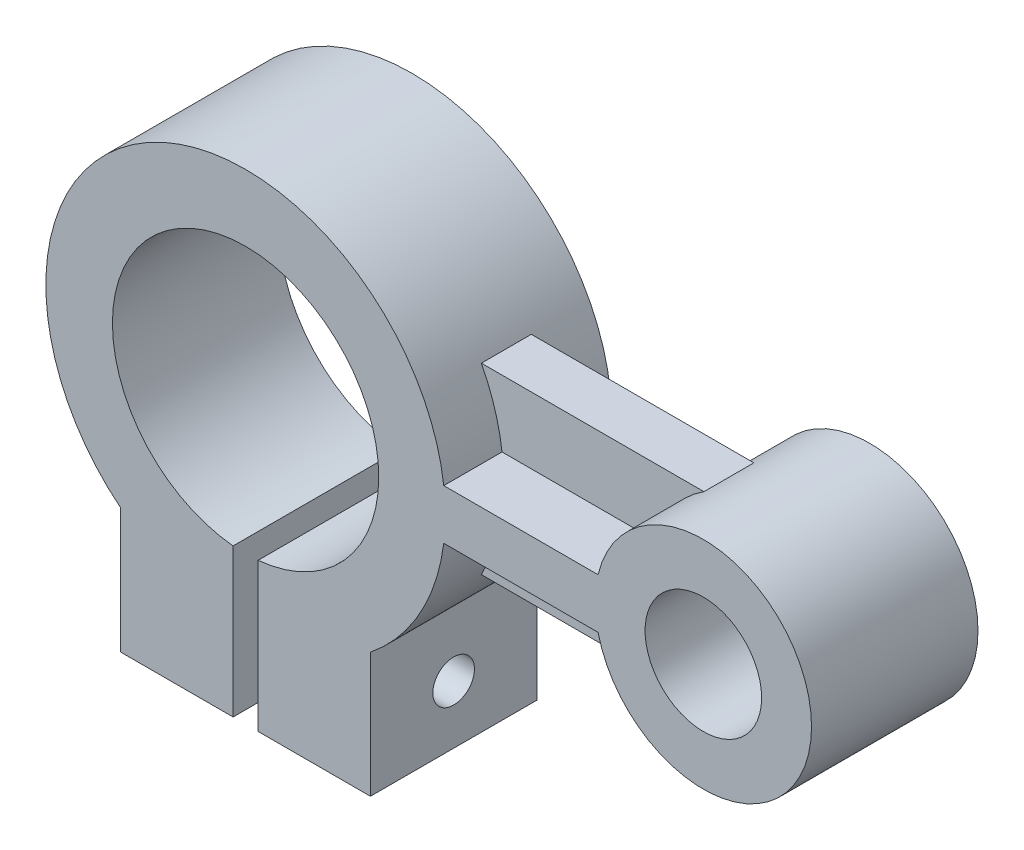
ISO-10303-21;
HEADER;
FILE_DESCRIPTION(('STEP AP214'),'2;1');
FILE_NAME('part.step','',(''),(''),'','','');
FILE_SCHEMA(('AUTOMOTIVE_DESIGN { 1 0 10303 214 1 1 1 1 }'));
ENDSEC;
DATA;
#1=APPLICATION_CONTEXT('core data for automotive mechanical design processes');
#2=APPLICATION_PROTOCOL_DEFINITION('international standard','automotive_design',2000,#1);
#3=PRODUCT_CONTEXT('',#1,'mechanical');
#4=PRODUCT('Part','Part','',(#3));
#5=PRODUCT_RELATED_PRODUCT_CATEGORY('part','',(#4));
#6=PRODUCT_DEFINITION_FORMATION('','',#4);
#7=PRODUCT_DEFINITION_CONTEXT('part definition',#1,'design');
#8=PRODUCT_DEFINITION('design','',#6,#7);
#9=PRODUCT_DEFINITION_SHAPE('','',#8);
#10=(LENGTH_UNIT() NAMED_UNIT(*) SI_UNIT(.MILLI.,.METRE.));
#11=(NAMED_UNIT(*) PLANE_ANGLE_UNIT() SI_UNIT($,.RADIAN.));
#12=(NAMED_UNIT(*) SI_UNIT($,.STERADIAN.) SOLID_ANGLE_UNIT());
#13=UNCERTAINTY_MEASURE_WITH_UNIT(LENGTH_MEASURE(1.E-05),#10,'distance_accuracy_value','');
#14=(GEOMETRIC_REPRESENTATION_CONTEXT(3) GLOBAL_UNCERTAINTY_ASSIGNED_CONTEXT((#13)) GLOBAL_UNIT_ASSIGNED_CONTEXT((#10,
#11,#12)) REPRESENTATION_CONTEXT('',''));
#15=CARTESIAN_POINT('',(0.,0.,0.));
#16=DIRECTION('',(0.,0.,1.));
#17=DIRECTION('',(1.,0.,0.));
#18=AXIS2_PLACEMENT_3D('',#15,#16,#17);
#19=CARTESIAN_POINT('',(110.,0.,0.));
#20=DIRECTION('',(0.,0.,1.));
#21=DIRECTION('',(1.,0.,0.));
#22=AXIS2_PLACEMENT_3D('',#19,#20,#21);
#23=CYLINDRICAL_SURFACE('',#22,26.);
#24=DIRECTION('',(0.,0.,1.));
#25=VECTOR('',#24,1.);
#26=CARTESIAN_POINT('',(96.143593539449,-22.,0.));
#27=LINE('',#26,#25);
#28=CARTESIAN_POINT('',(96.143593539449,-22.,26.));
#29=VERTEX_POINT('',#28);
#30=CARTESIAN_POINT('',(96.143593539449,-22.,14.));
#31=VERTEX_POINT('',#30);
#32=EDGE_CURVE('E345',#29,#31,#27,.F.);
#33=ORIENTED_EDGE('',*,*,#32,.T.);
#34=CARTESIAN_POINT('',(110.,0.,14.));
#35=DIRECTION('',(0.,0.,1.));
#36=DIRECTION('',(1.,0.,0.));
#37=AXIS2_PLACEMENT_3D('',#34,#35,#36);
#38=CIRCLE('',#37,26.);
#39=CARTESIAN_POINT('',(84.701778718653,-6.,14.));
#40=VERTEX_POINT('',#39);
#41=EDGE_CURVE('E349',#31,#40,#38,.F.);
#42=ORIENTED_EDGE('',*,*,#41,.T.);
#43=DIRECTION('',(0.,0.,1.));
#44=VECTOR('',#43,1.);
#45=CARTESIAN_POINT('',(84.701778718653,-6.,0.));
#46=LINE('',#45,#44);
#47=CARTESIAN_POINT('',(84.701778718653,-6.,0.));
#48=VERTEX_POINT('',#47);
#49=EDGE_CURVE('E214',#48,#40,#46,.T.);
#50=ORIENTED_EDGE('',*,*,#49,.F.);
#51=CARTESIAN_POINT('',(110.,0.,0.));
#52=DIRECTION('',(0.,0.,1.));
#53=DIRECTION('',(1.,0.,0.));
#54=AXIS2_PLACEMENT_3D('',#51,#52,#53);
#55=CIRCLE('',#54,26.);
#56=CARTESIAN_POINT('',(84.701778718653,6.,0.));
#57=VERTEX_POINT('',#56);
#58=EDGE_CURVE('E309',#48,#57,#55,.T.);
#59=ORIENTED_EDGE('',*,*,#58,.T.);
#60=DIRECTION('',(0.,0.,1.));
#61=VECTOR('',#60,1.);
#62=CARTESIAN_POINT('',(84.701778718653,6.,0.));
#63=LINE('',#62,#61);
#64=CARTESIAN_POINT('',(84.701778718653,6.,14.));
#65=VERTEX_POINT('',#64);
#66=EDGE_CURVE('E217',#57,#65,#63,.T.);
#67=ORIENTED_EDGE('',*,*,#66,.T.);
#68=CARTESIAN_POINT('',(110.,0.,14.));
#69=DIRECTION('',(0.,0.,1.));
#70=DIRECTION('',(1.,0.,0.));
#71=AXIS2_PLACEMENT_3D('',#68,#69,#70);
#72=CIRCLE('',#71,26.);
#73=CARTESIAN_POINT('',(96.143593539449,22.,14.));
#74=VERTEX_POINT('',#73);
#75=EDGE_CURVE('E286',#65,#74,#72,.F.);
#76=ORIENTED_EDGE('',*,*,#75,.T.);
#77=DIRECTION('',(0.,0.,1.));
#78=VECTOR('',#77,1.);
#79=CARTESIAN_POINT('',(96.143593539449,22.,0.));
#80=LINE('',#79,#78);
#81=CARTESIAN_POINT('',(96.143593539449,22.,26.));
#82=VERTEX_POINT('',#81);
#83=EDGE_CURVE('E278',#74,#82,#80,.T.);
#84=ORIENTED_EDGE('',*,*,#83,.T.);
#85=CARTESIAN_POINT('',(110.,0.,26.));
#86=DIRECTION('',(0.,0.,-1.));
#87=DIRECTION('',(-1.,0.,0.));
#88=AXIS2_PLACEMENT_3D('',#85,#86,#87);
#89=CIRCLE('',#88,26.);
#90=CARTESIAN_POINT('',(84.701778718653,6.,26.));
#91=VERTEX_POINT('',#90);
#92=EDGE_CURVE('E188',#82,#91,#89,.F.);
#93=ORIENTED_EDGE('',*,*,#92,.T.);
#94=CARTESIAN_POINT('',(84.701778718653,6.,40.));
#95=VERTEX_POINT('',#94);
#96=EDGE_CURVE('E216',#91,#95,#63,.T.);
#97=ORIENTED_EDGE('',*,*,#96,.T.);
#98=CARTESIAN_POINT('',(110.,0.,40.));
#99=DIRECTION('',(0.,0.,1.));
#100=DIRECTION('',(1.,0.,0.));
#101=AXIS2_PLACEMENT_3D('',#98,#99,#100);
#102=CIRCLE('',#101,26.);
#103=CARTESIAN_POINT('',(84.701778718653,-6.,40.));
#104=VERTEX_POINT('',#103);
#105=EDGE_CURVE('E321',#104,#95,#102,.T.);
#106=ORIENTED_EDGE('',*,*,#105,.F.);
#107=CARTESIAN_POINT('',(84.701778718653,-6.,26.));
#108=VERTEX_POINT('',#107);
#109=EDGE_CURVE('E206',#108,#104,#46,.T.);
#110=ORIENTED_EDGE('',*,*,#109,.F.);
#111=CARTESIAN_POINT('',(110.,0.,26.));
#112=DIRECTION('',(0.,0.,-1.));
#113=DIRECTION('',(-1.,0.,0.));
#114=AXIS2_PLACEMENT_3D('',#111,#112,#113);
#115=CIRCLE('',#114,26.);
#116=EDGE_CURVE('E64',#108,#29,#115,.F.);
#117=ORIENTED_EDGE('',*,*,#116,.T.);
#118=EDGE_LOOP('',(#33,#42,#50,#59,#67,#76,#84,#93,#97,#106,#110,#117));
#119=FACE_BOUND('',#118,.T.);
#120=ADVANCED_FACE('F50',(#119),#23,.T.);
#121=CARTESIAN_POINT('',(0.,0.,40.));
#122=DIRECTION('',(0.,0.,-1.));
#123=DIRECTION('',(-1.,0.,0.));
#124=AXIS2_PLACEMENT_3D('',#121,#122,#123);
#125=CYLINDRICAL_SURFACE('',#124,48.);
#126=CARTESIAN_POINT('',(0.,0.,14.));
#127=DIRECTION('',(0.,0.,1.));
#128=DIRECTION('',(1.,0.,0.));
#129=AXIS2_PLACEMENT_3D('',#126,#127,#128);
#130=CIRCLE('',#129,48.);
#131=CARTESIAN_POINT('',(42.6614580154031,-22.,14.));
#132=VERTEX_POINT('',#131);
#133=CARTESIAN_POINT('',(47.6235235991626,-6.,14.));
#134=VERTEX_POINT('',#133);
#135=EDGE_CURVE('E297',#132,#134,#130,.T.);
#136=ORIENTED_EDGE('',*,*,#135,.F.);
#137=DIRECTION('',(0.,0.,-1.));
#138=VECTOR('',#137,1.);
#139=CARTESIAN_POINT('',(42.6614580154031,-22.,40.));
#140=LINE('',#139,#138);
#141=CARTESIAN_POINT('',(42.6614580154031,-22.,26.));
#142=VERTEX_POINT('',#141);
#143=EDGE_CURVE('E11',#142,#132,#140,.T.);
#144=ORIENTED_EDGE('',*,*,#143,.F.);
#145=CARTESIAN_POINT('',(0.,0.,26.));
#146=DIRECTION('',(0.,0.,-1.));
#147=DIRECTION('',(-1.,0.,0.));
#148=AXIS2_PLACEMENT_3D('',#145,#146,#147);
#149=CIRCLE('',#148,48.);
#150=CARTESIAN_POINT('',(47.6235235991626,-6.,26.));
#151=VERTEX_POINT('',#150);
#152=EDGE_CURVE('E184',#151,#142,#149,.T.);
#153=ORIENTED_EDGE('',*,*,#152,.F.);
#154=DIRECTION('',(0.,0.,1.));
#155=VECTOR('',#154,1.);
#156=CARTESIAN_POINT('',(47.6235235991626,-6.00000000000002,0.));
#157=LINE('',#156,#155);
#158=CARTESIAN_POINT('',(47.6235235991626,-6.00000000000001,40.));
#159=VERTEX_POINT('',#158);
#160=EDGE_CURVE('E197',#151,#159,#157,.T.);
#161=ORIENTED_EDGE('',*,*,#160,.T.);
#162=CARTESIAN_POINT('',(0.,0.,40.));
#163=DIRECTION('',(0.,0.,1.));
#164=DIRECTION('',(1.,0.,0.));
#165=AXIS2_PLACEMENT_3D('',#162,#163,#164);
#166=CIRCLE('',#165,48.);
#167=CARTESIAN_POINT('',(30.,-37.4699879903904,40.));
#168=VERTEX_POINT('',#167);
#169=EDGE_CURVE('E279',#168,#159,#166,.T.);
#170=ORIENTED_EDGE('',*,*,#169,.F.);
#171=DIRECTION('',(0.,0.,1.));
#172=VECTOR('',#171,1.);
#173=CARTESIAN_POINT('',(30.,-37.4699879903904,0.));
#174=LINE('',#173,#172);
#175=CARTESIAN_POINT('',(30.,-37.4699879903904,0.));
#176=VERTEX_POINT('',#175);
#177=EDGE_CURVE('E267',#176,#168,#174,.T.);
#178=ORIENTED_EDGE('',*,*,#177,.F.);
#179=CARTESIAN_POINT('',(0.,0.,0.));
#180=DIRECTION('',(0.,0.,1.));
#181=DIRECTION('',(1.,0.,0.));
#182=AXIS2_PLACEMENT_3D('',#179,#180,#181);
#183=CIRCLE('',#182,48.);
#184=CARTESIAN_POINT('',(47.6235235991626,-6.00000000000001,0.));
#185=VERTEX_POINT('',#184);
#186=EDGE_CURVE('E284',#176,#185,#183,.T.);
#187=ORIENTED_EDGE('',*,*,#186,.T.);
#188=EDGE_CURVE('E203',#185,#134,#157,.T.);
#189=ORIENTED_EDGE('',*,*,#188,.T.);
#190=EDGE_LOOP('',(#136,#144,#153,#161,#170,#178,#187,#189));
#191=FACE_BOUND('',#190,.T.);
#192=ADVANCED_FACE('F193',(#191),#125,.T.);
#193=CARTESIAN_POINT('',(47.6235235991626,-6.,0.));
#194=DIRECTION('',(0.,-1.,0.));
#195=DIRECTION('',(1.,0.,0.));
#196=AXIS2_PLACEMENT_3D('',#193,#194,#195);
#197=PLANE('',#196);
#198=ORIENTED_EDGE('',*,*,#49,.T.);
#199=DIRECTION('',(-1.,0.,0.));
#200=VECTOR('',#199,1.);
#201=CARTESIAN_POINT('',(47.6235235991626,-6.,14.));
#202=LINE('',#201,#200);
#203=EDGE_CURVE('E57',#40,#134,#202,.T.);
#204=ORIENTED_EDGE('',*,*,#203,.T.);
#205=ORIENTED_EDGE('',*,*,#188,.F.);
#206=DIRECTION('',(1.,0.,0.));
#207=VECTOR('',#206,1.);
#208=CARTESIAN_POINT('',(47.6235235991626,-6.,0.));
#209=LINE('',#208,#207);
#210=EDGE_CURVE('E310',#185,#48,#209,.T.);
#211=ORIENTED_EDGE('',*,*,#210,.T.);
#212=EDGE_LOOP('',(#198,#204,#205,#211));
#213=FACE_BOUND('',#212,.T.);
#214=ADVANCED_FACE('F294',(#213),#197,.T.);
#215=ORIENTED_EDGE('',*,*,#160,.F.);
#216=DIRECTION('',(1.,0.,0.));
#217=VECTOR('',#216,1.);
#218=CARTESIAN_POINT('',(47.6235235991626,-6.,26.));
#219=LINE('',#218,#217);
#220=EDGE_CURVE('E185',#151,#108,#219,.T.);
#221=ORIENTED_EDGE('',*,*,#220,.T.);
#222=ORIENTED_EDGE('',*,*,#109,.T.);
#223=DIRECTION('',(1.,0.,0.));
#224=VECTOR('',#223,1.);
#225=CARTESIAN_POINT('',(47.6235235991626,-6.,40.));
#226=LINE('',#225,#224);
#227=EDGE_CURVE('E204',#159,#104,#226,.T.);
#228=ORIENTED_EDGE('',*,*,#227,.F.);
#229=EDGE_LOOP('',(#215,#221,#222,#228));
#230=FACE_BOUND('',#229,.T.);
#231=ADVANCED_FACE('F201',(#230),#197,.T.);
#232=CARTESIAN_POINT('',(0.,0.,26.));
#233=DIRECTION('',(0.,0.,-1.));
#234=DIRECTION('',(-1.,0.,0.));
#235=AXIS2_PLACEMENT_3D('',#232,#233,#234);
#236=CIRCLE('',#235,48.);
#237=CARTESIAN_POINT('',(42.6614580154031,22.,26.));
#238=VERTEX_POINT('',#237);
#239=CARTESIAN_POINT('',(47.6235235991626,6.,26.));
#240=VERTEX_POINT('',#239);
#241=EDGE_CURVE('E326',#238,#240,#236,.T.);
#242=ORIENTED_EDGE('',*,*,#241,.F.);
#243=DIRECTION('',(0.,0.,-1.));
#244=VECTOR('',#243,1.);
#245=CARTESIAN_POINT('',(42.6614580154031,22.,40.));
#246=LINE('',#245,#244);
#247=CARTESIAN_POINT('',(42.6614580154031,22.,14.));
#248=VERTEX_POINT('',#247);
#249=EDGE_CURVE('E335',#248,#238,#246,.F.);
#250=ORIENTED_EDGE('',*,*,#249,.F.);
#251=CARTESIAN_POINT('',(0.,0.,14.));
#252=DIRECTION('',(0.,0.,1.));
#253=DIRECTION('',(1.,0.,0.));
#254=AXIS2_PLACEMENT_3D('',#251,#252,#253);
#255=CIRCLE('',#254,48.);
#256=CARTESIAN_POINT('',(47.6235235991626,6.,14.));
#257=VERTEX_POINT('',#256);
#258=EDGE_CURVE('E331',#257,#248,#255,.T.);
#259=ORIENTED_EDGE('',*,*,#258,.F.);
#260=DIRECTION('',(0.,0.,1.));
#261=VECTOR('',#260,1.);
#262=CARTESIAN_POINT('',(47.6235235991626,6.,0.));
#263=LINE('',#262,#261);
#264=CARTESIAN_POINT('',(47.6235235991626,6.,0.));
#265=VERTEX_POINT('',#264);
#266=EDGE_CURVE('E205',#265,#257,#263,.T.);
#267=ORIENTED_EDGE('',*,*,#266,.F.);
#268=CARTESIAN_POINT('',(-30.,-37.4699879903904,0.));
#269=VERTEX_POINT('',#268);
#270=EDGE_CURVE('E270',#265,#269,#183,.T.);
#271=ORIENTED_EDGE('',*,*,#270,.T.);
#272=DIRECTION('',(0.,0.,1.));
#273=VECTOR('',#272,1.);
#274=CARTESIAN_POINT('',(-30.,-37.4699879903904,0.));
#275=LINE('',#274,#273);
#276=CARTESIAN_POINT('',(-30.,-37.4699879903904,40.));
#277=VERTEX_POINT('',#276);
#278=EDGE_CURVE('E259',#269,#277,#275,.T.);
#279=ORIENTED_EDGE('',*,*,#278,.T.);
#280=CARTESIAN_POINT('',(47.6235235991626,6.,40.));
#281=VERTEX_POINT('',#280);
#282=EDGE_CURVE('E282',#281,#277,#166,.T.);
#283=ORIENTED_EDGE('',*,*,#282,.F.);
#284=EDGE_CURVE('E208',#240,#281,#263,.T.);
#285=ORIENTED_EDGE('',*,*,#284,.F.);
#286=EDGE_LOOP('',(#242,#250,#259,#267,#271,#279,#283,#285));
#287=FACE_BOUND('',#286,.T.);
#288=ADVANCED_FACE('F47',(#287),#125,.T.);
#289=CARTESIAN_POINT('',(47.6235235991626,6.,0.));
#290=DIRECTION('',(0.,1.,0.));
#291=DIRECTION('',(-1.,0.,0.));
#292=AXIS2_PLACEMENT_3D('',#289,#290,#291);
#293=PLANE('',#292);
#294=ORIENTED_EDGE('',*,*,#96,.F.);
#295=DIRECTION('',(1.,0.,0.));
#296=VECTOR('',#295,1.);
#297=CARTESIAN_POINT('',(110.350889359326,6.,26.));
#298=LINE('',#297,#296);
#299=EDGE_CURVE('E338',#240,#91,#298,.T.);
#300=ORIENTED_EDGE('',*,*,#299,.F.);
#301=ORIENTED_EDGE('',*,*,#284,.T.);
#302=DIRECTION('',(-1.,0.,0.));
#303=VECTOR('',#302,1.);
#304=CARTESIAN_POINT('',(47.6235235991626,6.,40.));
#305=LINE('',#304,#303);
#306=EDGE_CURVE('E320',#95,#281,#305,.T.);
#307=ORIENTED_EDGE('',*,*,#306,.F.);
#308=EDGE_LOOP('',(#294,#300,#301,#307));
#309=FACE_BOUND('',#308,.T.);
#310=ADVANCED_FACE('F405',(#309),#293,.T.);
#311=ORIENTED_EDGE('',*,*,#266,.T.);
#312=DIRECTION('',(-1.,0.,0.));
#313=VECTOR('',#312,1.);
#314=CARTESIAN_POINT('',(39.2683528470453,6.,14.));
#315=LINE('',#314,#313);
#316=EDGE_CURVE('E336',#65,#257,#315,.T.);
#317=ORIENTED_EDGE('',*,*,#316,.F.);
#318=ORIENTED_EDGE('',*,*,#66,.F.);
#319=DIRECTION('',(-1.,0.,0.));
#320=VECTOR('',#319,1.);
#321=CARTESIAN_POINT('',(47.6235235991626,6.,0.));
#322=LINE('',#321,#320);
#323=EDGE_CURVE('E311',#57,#265,#322,.T.);
#324=ORIENTED_EDGE('',*,*,#323,.T.);
#325=EDGE_LOOP('',(#311,#317,#318,#324));
#326=FACE_BOUND('',#325,.T.);
#327=ADVANCED_FACE('F403',(#326),#293,.T.);
#328=CARTESIAN_POINT('',(-30.,-67.4699879903904,0.));
#329=DIRECTION('',(0.,-1.,0.));
#330=DIRECTION('',(0.,0.,-1.));
#331=AXIS2_PLACEMENT_3D('',#328,#329,#330);
#332=PLANE('',#331);
#333=DIRECTION('',(0.,0.,1.));
#334=VECTOR('',#333,1.);
#335=CARTESIAN_POINT('',(3.00000000000001,-67.4699879903904,0.));
#336=LINE('',#335,#334);
#337=CARTESIAN_POINT('',(3.00000000000001,-67.4699879903904,0.));
#338=VERTEX_POINT('',#337);
#339=CARTESIAN_POINT('',(3.00000000000001,-67.4699879903904,40.));
#340=VERTEX_POINT('',#339);
#341=EDGE_CURVE('E241',#338,#340,#336,.T.);
#342=ORIENTED_EDGE('',*,*,#341,.F.);
#343=DIRECTION('',(1.,0.,0.));
#344=VECTOR('',#343,1.);
#345=CARTESIAN_POINT('',(-30.,-67.4699879903904,0.));
#346=LINE('',#345,#344);
#347=CARTESIAN_POINT('',(30.,-67.4699879903904,0.));
#348=VERTEX_POINT('',#347);
#349=EDGE_CURVE('E249',#338,#348,#346,.T.);
#350=ORIENTED_EDGE('',*,*,#349,.T.);
#351=DIRECTION('',(0.,0.,1.));
#352=VECTOR('',#351,1.);
#353=CARTESIAN_POINT('',(30.,-67.4699879903904,0.));
#354=LINE('',#353,#352);
#355=CARTESIAN_POINT('',(30.,-67.4699879903904,40.));
#356=VERTEX_POINT('',#355);
#357=EDGE_CURVE('E272',#348,#356,#354,.T.);
#358=ORIENTED_EDGE('',*,*,#357,.T.);
#359=DIRECTION('',(1.,0.,0.));
#360=VECTOR('',#359,1.);
#361=CARTESIAN_POINT('',(-30.,-67.4699879903904,40.));
#362=LINE('',#361,#360);
#363=EDGE_CURVE('E262',#340,#356,#362,.T.);
#364=ORIENTED_EDGE('',*,*,#363,.F.);
#365=EDGE_LOOP('',(#342,#350,#358,#364));
#366=FACE_BOUND('',#365,.T.);
#367=ADVANCED_FACE('F428',(#366),#332,.T.);
#368=CARTESIAN_POINT('',(0.,0.,40.));
#369=DIRECTION('',(0.,0.,1.));
#370=DIRECTION('',(1.,0.,0.));
#371=AXIS2_PLACEMENT_3D('',#368,#369,#370);
#372=PLANE('',#371);
#373=CARTESIAN_POINT('',(110.,0.,40.));
#374=DIRECTION('',(0.,0.,1.));
#375=DIRECTION('',(1.,0.,0.));
#376=AXIS2_PLACEMENT_3D('',#373,#374,#375);
#377=CIRCLE('',#376,14.);
#378=CARTESIAN_POINT('',(124.,0.,40.));
#379=VERTEX_POINT('',#378);
#380=EDGE_CURVE('E358',#379,#379,#377,.T.);
#381=ORIENTED_EDGE('',*,*,#380,.F.);
#382=EDGE_LOOP('',(#381));
#383=FACE_BOUND('',#382,.T.);
#384=DIRECTION('',(0.,1.,0.));
#385=VECTOR('',#384,1.);
#386=CARTESIAN_POINT('',(3.00000000000001,-67.4699879903904,40.));
#387=LINE('',#386,#385);
#388=CARTESIAN_POINT('',(3.00000000000001,-31.859064644148,40.));
#389=VERTEX_POINT('',#388);
#390=EDGE_CURVE('E223',#340,#389,#387,.T.);
#391=ORIENTED_EDGE('',*,*,#390,.F.);
#392=ORIENTED_EDGE('',*,*,#363,.T.);
#393=DIRECTION('',(0.,1.,0.));
#394=VECTOR('',#393,1.);
#395=CARTESIAN_POINT('',(30.,-67.4699879903904,40.));
#396=LINE('',#395,#394);
#397=EDGE_CURVE('E252',#356,#168,#396,.T.);
#398=ORIENTED_EDGE('',*,*,#397,.T.);
#399=ORIENTED_EDGE('',*,*,#169,.T.);
#400=ORIENTED_EDGE('',*,*,#227,.T.);
#401=ORIENTED_EDGE('',*,*,#105,.T.);
#402=ORIENTED_EDGE('',*,*,#306,.T.);
#403=ORIENTED_EDGE('',*,*,#282,.T.);
#404=DIRECTION('',(0.,-1.,0.));
#405=VECTOR('',#404,1.);
#406=CARTESIAN_POINT('',(-30.,-67.4699879903904,40.));
#407=LINE('',#406,#405);
#408=CARTESIAN_POINT('',(-30.,-67.4699879903904,40.));
#409=VERTEX_POINT('',#408);
#410=EDGE_CURVE('E239',#277,#409,#407,.T.);
#411=ORIENTED_EDGE('',*,*,#410,.T.);
#412=CARTESIAN_POINT('',(-2.99999999999999,-67.4699879903904,40.));
#413=VERTEX_POINT('',#412);
#414=EDGE_CURVE('E264',#409,#413,#362,.T.);
#415=ORIENTED_EDGE('',*,*,#414,.T.);
#416=DIRECTION('',(0.,-1.,0.));
#417=VECTOR('',#416,1.);
#418=CARTESIAN_POINT('',(-2.99999999999999,-31.859064644148,40.));
#419=LINE('',#418,#417);
#420=CARTESIAN_POINT('',(-2.99999999999999,-31.859064644148,40.));
#421=VERTEX_POINT('',#420);
#422=EDGE_CURVE('E234',#421,#413,#419,.T.);
#423=ORIENTED_EDGE('',*,*,#422,.F.);
#424=CARTESIAN_POINT('',(0.,0.,40.));
#425=DIRECTION('',(0.,0.,1.));
#426=DIRECTION('',(1.,0.,0.));
#427=AXIS2_PLACEMENT_3D('',#424,#425,#426);
#428=CIRCLE('',#427,32.);
#429=EDGE_CURVE('E233',#389,#421,#428,.T.);
#430=ORIENTED_EDGE('',*,*,#429,.F.);
#431=EDGE_LOOP('',(#391,#392,#398,#399,#400,#401,#402,#403,#411,#415,#423,#430));
#432=FACE_BOUND('',#431,.T.);
#433=ADVANCED_FACE('F324',(#383,#432),#372,.T.);
#434=CARTESIAN_POINT('',(0.,0.,0.));
#435=DIRECTION('',(0.,0.,1.));
#436=DIRECTION('',(1.,0.,0.));
#437=AXIS2_PLACEMENT_3D('',#434,#435,#436);
#438=PLANE('',#437);
#439=CARTESIAN_POINT('',(110.,0.,0.));
#440=DIRECTION('',(0.,0.,1.));
#441=DIRECTION('',(1.,0.,0.));
#442=AXIS2_PLACEMENT_3D('',#439,#440,#441);
#443=CIRCLE('',#442,14.);
#444=CARTESIAN_POINT('',(124.,0.,0.));
#445=VERTEX_POINT('',#444);
#446=EDGE_CURVE('E355',#445,#445,#443,.T.);
#447=ORIENTED_EDGE('',*,*,#446,.T.);
#448=EDGE_LOOP('',(#447));
#449=FACE_BOUND('',#448,.T.);
#450=ORIENTED_EDGE('',*,*,#349,.F.);
#451=DIRECTION('',(0.,1.,0.));
#452=VECTOR('',#451,1.);
#453=CARTESIAN_POINT('',(3.00000000000001,-67.4699879903904,0.));
#454=LINE('',#453,#452);
#455=CARTESIAN_POINT('',(3.00000000000001,-31.859064644148,0.));
#456=VERTEX_POINT('',#455);
#457=EDGE_CURVE('E227',#338,#456,#454,.T.);
#458=ORIENTED_EDGE('',*,*,#457,.T.);
#459=CARTESIAN_POINT('',(0.,0.,0.));
#460=DIRECTION('',(0.,0.,1.));
#461=DIRECTION('',(1.,0.,0.));
#462=AXIS2_PLACEMENT_3D('',#459,#460,#461);
#463=CIRCLE('',#462,32.);
#464=CARTESIAN_POINT('',(-2.99999999999999,-31.859064644148,0.));
#465=VERTEX_POINT('',#464);
#466=EDGE_CURVE('E218',#456,#465,#463,.T.);
#467=ORIENTED_EDGE('',*,*,#466,.T.);
#468=DIRECTION('',(0.,-1.,0.));
#469=VECTOR('',#468,1.);
#470=CARTESIAN_POINT('',(-2.99999999999999,-31.859064644148,0.));
#471=LINE('',#470,#469);
#472=CARTESIAN_POINT('',(-2.99999999999999,-67.4699879903904,0.));
#473=VERTEX_POINT('',#472);
#474=EDGE_CURVE('E224',#465,#473,#471,.T.);
#475=ORIENTED_EDGE('',*,*,#474,.T.);
#476=CARTESIAN_POINT('',(-30.,-67.4699879903904,0.));
#477=VERTEX_POINT('',#476);
#478=EDGE_CURVE('E255',#477,#473,#346,.T.);
#479=ORIENTED_EDGE('',*,*,#478,.F.);
#480=DIRECTION('',(0.,-1.,0.));
#481=VECTOR('',#480,1.);
#482=CARTESIAN_POINT('',(-30.,-67.4699879903904,0.));
#483=LINE('',#482,#481);
#484=EDGE_CURVE('E250',#269,#477,#483,.T.);
#485=ORIENTED_EDGE('',*,*,#484,.F.);
#486=ORIENTED_EDGE('',*,*,#270,.F.);
#487=ORIENTED_EDGE('',*,*,#323,.F.);
#488=ORIENTED_EDGE('',*,*,#58,.F.);
#489=ORIENTED_EDGE('',*,*,#210,.F.);
#490=ORIENTED_EDGE('',*,*,#186,.F.);
#491=DIRECTION('',(0.,1.,0.));
#492=VECTOR('',#491,1.);
#493=CARTESIAN_POINT('',(30.,-67.4699879903904,0.));
#494=LINE('',#493,#492);
#495=EDGE_CURVE('E253',#348,#176,#494,.T.);
#496=ORIENTED_EDGE('',*,*,#495,.F.);
#497=EDGE_LOOP('',(#450,#458,#467,#475,#479,#485,#486,#487,#488,#489,#490,#496));
#498=FACE_BOUND('',#497,.T.);
#499=ADVANCED_FACE('F304',(#449,#498),#438,.F.);
#500=CARTESIAN_POINT('',(30.,-67.4699879903904,0.));
#501=DIRECTION('',(1.,0.,0.));
#502=DIRECTION('',(0.,0.,-1.));
#503=AXIS2_PLACEMENT_3D('',#500,#501,#502);
#504=PLANE('',#503);
#505=CARTESIAN_POINT('',(30.,-53.4699879903904,20.));
#506=DIRECTION('',(1.,0.,0.));
#507=DIRECTION('',(0.,0.,-1.));
#508=AXIS2_PLACEMENT_3D('',#505,#506,#507);
#509=CIRCLE('',#508,5.00000000000001);
#510=CARTESIAN_POINT('',(30.,-53.4699879903904,15.));
#511=VERTEX_POINT('',#510);
#512=EDGE_CURVE('E370',#511,#511,#509,.T.);
#513=ORIENTED_EDGE('',*,*,#512,.F.);
#514=EDGE_LOOP('',(#513));
#515=FACE_BOUND('',#514,.T.);
#516=ORIENTED_EDGE('',*,*,#397,.F.);
#517=ORIENTED_EDGE('',*,*,#357,.F.);
#518=ORIENTED_EDGE('',*,*,#495,.T.);
#519=ORIENTED_EDGE('',*,*,#177,.T.);
#520=EDGE_LOOP('',(#516,#517,#518,#519));
#521=FACE_BOUND('',#520,.T.);
#522=ADVANCED_FACE('F419',(#515,#521),#504,.T.);
#523=DIRECTION('',(0.,0.,1.));
#524=VECTOR('',#523,1.);
#525=CARTESIAN_POINT('',(-2.99999999999999,-67.4699879903904,0.));
#526=LINE('',#525,#524);
#527=EDGE_CURVE('E243',#473,#413,#526,.T.);
#528=ORIENTED_EDGE('',*,*,#527,.T.);
#529=ORIENTED_EDGE('',*,*,#414,.F.);
#530=DIRECTION('',(0.,0.,1.));
#531=VECTOR('',#530,1.);
#532=CARTESIAN_POINT('',(-30.,-67.4699879903904,0.));
#533=LINE('',#532,#531);
#534=EDGE_CURVE('E274',#477,#409,#533,.T.);
#535=ORIENTED_EDGE('',*,*,#534,.F.);
#536=ORIENTED_EDGE('',*,*,#478,.T.);
#537=EDGE_LOOP('',(#528,#529,#535,#536));
#538=FACE_BOUND('',#537,.T.);
#539=ADVANCED_FACE('F423',(#538),#332,.T.);
#540=CARTESIAN_POINT('',(-30.,-67.4699879903904,0.));
#541=DIRECTION('',(-1.,0.,0.));
#542=DIRECTION('',(0.,0.,1.));
#543=AXIS2_PLACEMENT_3D('',#540,#541,#542);
#544=PLANE('',#543);
#545=CARTESIAN_POINT('',(-30.,-53.4699879903904,20.));
#546=DIRECTION('',(-1.,0.,0.));
#547=DIRECTION('',(0.,0.,1.));
#548=AXIS2_PLACEMENT_3D('',#545,#546,#547);
#549=CIRCLE('',#548,5.00000000000001);
#550=CARTESIAN_POINT('',(-30.,-53.4699879903904,25.));
#551=VERTEX_POINT('',#550);
#552=EDGE_CURVE('E360',#551,#551,#549,.T.);
#553=ORIENTED_EDGE('',*,*,#552,.F.);
#554=EDGE_LOOP('',(#553));
#555=FACE_BOUND('',#554,.T.);
#556=ORIENTED_EDGE('',*,*,#410,.F.);
#557=ORIENTED_EDGE('',*,*,#278,.F.);
#558=ORIENTED_EDGE('',*,*,#484,.T.);
#559=ORIENTED_EDGE('',*,*,#534,.T.);
#560=EDGE_LOOP('',(#556,#557,#558,#559));
#561=FACE_BOUND('',#560,.T.);
#562=ADVANCED_FACE('F416',(#555,#561),#544,.T.);
#563=CARTESIAN_POINT('',(0.,0.,0.));
#564=DIRECTION('',(0.,0.,1.));
#565=DIRECTION('',(1.,0.,0.));
#566=AXIS2_PLACEMENT_3D('',#563,#564,#565);
#567=CYLINDRICAL_SURFACE('',#566,32.);
#568=ORIENTED_EDGE('',*,*,#429,.T.);
#569=DIRECTION('',(0.,0.,1.));
#570=VECTOR('',#569,1.);
#571=CARTESIAN_POINT('',(-2.99999999999999,-31.859064644148,0.));
#572=LINE('',#571,#570);
#573=EDGE_CURVE('E229',#465,#421,#572,.T.);
#574=ORIENTED_EDGE('',*,*,#573,.F.);
#575=ORIENTED_EDGE('',*,*,#466,.F.);
#576=DIRECTION('',(0.,0.,1.));
#577=VECTOR('',#576,1.);
#578=CARTESIAN_POINT('',(3.00000000000001,-31.859064644148,0.));
#579=LINE('',#578,#577);
#580=EDGE_CURVE('E238',#456,#389,#579,.T.);
#581=ORIENTED_EDGE('',*,*,#580,.T.);
#582=EDGE_LOOP('',(#568,#574,#575,#581));
#583=FACE_BOUND('',#582,.T.);
#584=ADVANCED_FACE('F408',(#583),#567,.F.);
#585=CARTESIAN_POINT('',(3.00000000000001,-67.4699879903904,0.));
#586=DIRECTION('',(1.,0.,0.));
#587=DIRECTION('',(0.,0.,-1.));
#588=AXIS2_PLACEMENT_3D('',#585,#586,#587);
#589=PLANE('',#588);
#590=CARTESIAN_POINT('',(3.,-53.4699879903904,20.));
#591=DIRECTION('',(1.,0.,0.));
#592=DIRECTION('',(0.,0.,-1.));
#593=AXIS2_PLACEMENT_3D('',#590,#591,#592);
#594=CIRCLE('',#593,5.00000000000001);
#595=CARTESIAN_POINT('',(3.,-53.4699879903904,15.));
#596=VERTEX_POINT('',#595);
#597=EDGE_CURVE('E364',#596,#596,#594,.T.);
#598=ORIENTED_EDGE('',*,*,#597,.T.);
#599=EDGE_LOOP('',(#598));
#600=FACE_BOUND('',#599,.T.);
#601=ORIENTED_EDGE('',*,*,#390,.T.);
#602=ORIENTED_EDGE('',*,*,#580,.F.);
#603=ORIENTED_EDGE('',*,*,#457,.F.);
#604=ORIENTED_EDGE('',*,*,#341,.T.);
#605=EDGE_LOOP('',(#601,#602,#603,#604));
#606=FACE_BOUND('',#605,.T.);
#607=ADVANCED_FACE('F410',(#600,#606),#589,.F.);
#608=CARTESIAN_POINT('',(-2.99999999999999,-31.859064644148,0.));
#609=DIRECTION('',(-1.,0.,0.));
#610=DIRECTION('',(0.,-1.,0.));
#611=AXIS2_PLACEMENT_3D('',#608,#609,#610);
#612=PLANE('',#611);
#613=CARTESIAN_POINT('',(-3.,-53.4699879903904,20.));
#614=DIRECTION('',(-1.,0.,0.));
#615=DIRECTION('',(0.,-1.,0.));
#616=AXIS2_PLACEMENT_3D('',#613,#614,#615);
#617=CIRCLE('',#616,5.00000000000001);
#618=CARTESIAN_POINT('',(-3.,-58.4699879903904,20.));
#619=VERTEX_POINT('',#618);
#620=EDGE_CURVE('E51',#619,#619,#617,.T.);
#621=ORIENTED_EDGE('',*,*,#620,.T.);
#622=EDGE_LOOP('',(#621));
#623=FACE_BOUND('',#622,.T.);
#624=ORIENTED_EDGE('',*,*,#422,.T.);
#625=ORIENTED_EDGE('',*,*,#527,.F.);
#626=ORIENTED_EDGE('',*,*,#474,.F.);
#627=ORIENTED_EDGE('',*,*,#573,.T.);
#628=EDGE_LOOP('',(#624,#625,#626,#627));
#629=FACE_BOUND('',#628,.T.);
#630=ADVANCED_FACE('F372',(#623,#629),#612,.F.);
#631=CARTESIAN_POINT('',(110.350889359326,22.,26.));
#632=DIRECTION('',(0.,0.,-1.));
#633=DIRECTION('',(-1.,0.,0.));
#634=AXIS2_PLACEMENT_3D('',#631,#632,#633);
#635=PLANE('',#634);
#636=DIRECTION('',(1.,0.,0.));
#637=VECTOR('',#636,1.);
#638=CARTESIAN_POINT('',(98.516804153608,22.,26.));
#639=LINE('',#638,#637);
#640=EDGE_CURVE('E71',#238,#82,#639,.T.);
#641=ORIENTED_EDGE('',*,*,#640,.F.);
#642=ORIENTED_EDGE('',*,*,#241,.T.);
#643=ORIENTED_EDGE('',*,*,#299,.T.);
#644=ORIENTED_EDGE('',*,*,#92,.F.);
#645=EDGE_LOOP('',(#641,#642,#643,#644));
#646=FACE_BOUND('',#645,.T.);
#647=ADVANCED_FACE('F399',(#646),#635,.F.);
#648=CARTESIAN_POINT('',(39.2683528470453,22.,14.));
#649=DIRECTION('',(0.,0.,1.));
#650=DIRECTION('',(1.,0.,0.));
#651=AXIS2_PLACEMENT_3D('',#648,#649,#650);
#652=PLANE('',#651);
#653=ORIENTED_EDGE('',*,*,#316,.T.);
#654=ORIENTED_EDGE('',*,*,#258,.T.);
#655=DIRECTION('',(-1.,0.,0.));
#656=VECTOR('',#655,1.);
#657=CARTESIAN_POINT('',(98.516804153608,22.,14.));
#658=LINE('',#657,#656);
#659=EDGE_CURVE('E340',#74,#248,#658,.T.);
#660=ORIENTED_EDGE('',*,*,#659,.F.);
#661=ORIENTED_EDGE('',*,*,#75,.F.);
#662=EDGE_LOOP('',(#653,#654,#660,#661));
#663=FACE_BOUND('',#662,.T.);
#664=ADVANCED_FACE('F538',(#663),#652,.F.);
#665=CARTESIAN_POINT('',(0.,22.,0.));
#666=DIRECTION('',(0.,-1.,0.));
#667=DIRECTION('',(1.,0.,0.));
#668=AXIS2_PLACEMENT_3D('',#665,#666,#667);
#669=PLANE('',#668);
#670=ORIENTED_EDGE('',*,*,#659,.T.);
#671=ORIENTED_EDGE('',*,*,#249,.T.);
#672=ORIENTED_EDGE('',*,*,#640,.T.);
#673=ORIENTED_EDGE('',*,*,#83,.F.);
#674=EDGE_LOOP('',(#670,#671,#672,#673));
#675=FACE_BOUND('',#674,.T.);
#676=ADVANCED_FACE('F508',(#675),#669,.F.);
#677=CARTESIAN_POINT('',(0.,-22.,0.));
#678=DIRECTION('',(0.,1.,0.));
#679=DIRECTION('',(-1.,0.,0.));
#680=AXIS2_PLACEMENT_3D('',#677,#678,#679);
#681=PLANE('',#680);
#682=ORIENTED_EDGE('',*,*,#32,.F.);
#683=DIRECTION('',(-1.,0.,0.));
#684=VECTOR('',#683,1.);
#685=CARTESIAN_POINT('',(38.2397339007508,-22.,26.));
#686=LINE('',#685,#684);
#687=EDGE_CURVE('E200',#29,#142,#686,.T.);
#688=ORIENTED_EDGE('',*,*,#687,.T.);
#689=ORIENTED_EDGE('',*,*,#143,.T.);
#690=DIRECTION('',(1.,0.,0.));
#691=VECTOR('',#690,1.);
#692=CARTESIAN_POINT('',(110.350889359326,-22.,14.));
#693=LINE('',#692,#691);
#694=EDGE_CURVE('E352',#132,#31,#693,.T.);
#695=ORIENTED_EDGE('',*,*,#694,.T.);
#696=EDGE_LOOP('',(#682,#688,#689,#695));
#697=FACE_BOUND('',#696,.T.);
#698=ADVANCED_FACE('F499',(#697),#681,.F.);
#699=CARTESIAN_POINT('',(110.350889359326,-22.,14.));
#700=DIRECTION('',(0.,0.,1.));
#701=DIRECTION('',(1.,0.,0.));
#702=AXIS2_PLACEMENT_3D('',#699,#700,#701);
#703=PLANE('',#702);
#704=ORIENTED_EDGE('',*,*,#41,.F.);
#705=ORIENTED_EDGE('',*,*,#694,.F.);
#706=ORIENTED_EDGE('',*,*,#135,.T.);
#707=ORIENTED_EDGE('',*,*,#203,.F.);
#708=EDGE_LOOP('',(#704,#705,#706,#707));
#709=FACE_BOUND('',#708,.T.);
#710=ADVANCED_FACE('F489',(#709),#703,.F.);
#711=CARTESIAN_POINT('',(38.2397339007508,-22.,26.));
#712=DIRECTION('',(0.,0.,-1.));
#713=DIRECTION('',(-1.,0.,0.));
#714=AXIS2_PLACEMENT_3D('',#711,#712,#713);
#715=PLANE('',#714);
#716=ORIENTED_EDGE('',*,*,#116,.F.);
#717=ORIENTED_EDGE('',*,*,#220,.F.);
#718=ORIENTED_EDGE('',*,*,#152,.T.);
#719=ORIENTED_EDGE('',*,*,#687,.F.);
#720=EDGE_LOOP('',(#716,#717,#718,#719));
#721=FACE_BOUND('',#720,.T.);
#722=ADVANCED_FACE('F183',(#721),#715,.F.);
#723=CARTESIAN_POINT('',(110.,0.,0.));
#724=DIRECTION('',(0.,0.,1.));
#725=DIRECTION('',(1.,0.,0.));
#726=AXIS2_PLACEMENT_3D('',#723,#724,#725);
#727=CYLINDRICAL_SURFACE('',#726,14.);
#728=ORIENTED_EDGE('',*,*,#446,.F.);
#729=EDGE_LOOP('',(#728));
#730=FACE_BOUND('',#729,.T.);
#731=ORIENTED_EDGE('',*,*,#380,.T.);
#732=EDGE_LOOP('',(#731));
#733=FACE_BOUND('',#732,.T.);
#734=ADVANCED_FACE('F379',(#730,#733),#727,.F.);
#735=CARTESIAN_POINT('',(-50.,-53.4699879903904,20.));
#736=DIRECTION('',(1.,0.,0.));
#737=DIRECTION('',(0.,0.,-1.));
#738=AXIS2_PLACEMENT_3D('',#735,#736,#737);
#739=CYLINDRICAL_SURFACE('',#738,5.00000000000001);
#740=ORIENTED_EDGE('',*,*,#552,.T.);
#741=EDGE_LOOP('',(#740));
#742=FACE_BOUND('',#741,.T.);
#743=ORIENTED_EDGE('',*,*,#620,.F.);
#744=EDGE_LOOP('',(#743));
#745=FACE_BOUND('',#744,.T.);
#746=ADVANCED_FACE('F380',(#742,#745),#739,.F.);
#747=ORIENTED_EDGE('',*,*,#512,.T.);
#748=EDGE_LOOP('',(#747));
#749=FACE_BOUND('',#748,.T.);
#750=ORIENTED_EDGE('',*,*,#597,.F.);
#751=EDGE_LOOP('',(#750));
#752=FACE_BOUND('',#751,.T.);
#753=ADVANCED_FACE('F378',(#749,#752),#739,.F.);
#754=CLOSED_SHELL('',(#120,#192,#214,#231,#288,#310,#327,#367,#433,#499,#522,#539,#562,#584,
#607,#630,#647,#664,#676,#698,#710,#722,#734,#746,#753));
#755=MANIFOLD_SOLID_BREP('B2',#754);
#756=ADVANCED_BREP_SHAPE_REPRESENTATION('',(#18,#755),#14);
#757=SHAPE_DEFINITION_REPRESENTATION(#9,#756);
ENDSEC;
END-ISO-10303-21;
